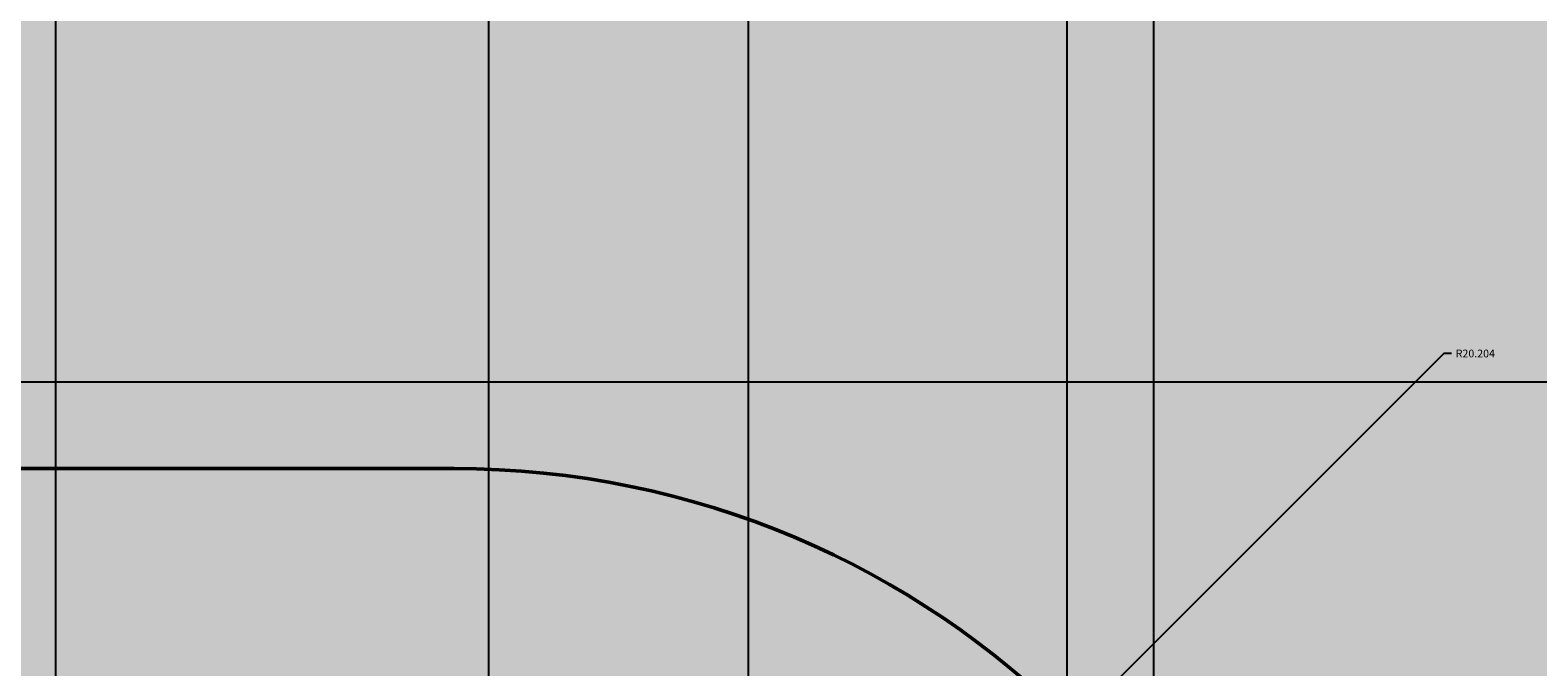
# Model space of a CAD drawing. Units: inches. Extents: x -12 to 334, y -10 to 186.
# Tile 56 of 77: x 222 to 257, y 96 to 111. Entities that reach past the tile are written whole.
import ezdxf

# ---------------------------------------------------------------- set-up
doc = ezdxf.new("R2010")
doc.units = ezdxf.units.IN
doc.header["$MEASUREMENT"] = 0
for name, color, linetype, lineweight in [('M-DIMS', 2, 'Continuous', 18), ('M-EQPM', 7, 'Continuous', 50), ('M-EQPM-PATT', 8, 'Continuous', 18)]:
    doc.layers.add(name, color=color, linetype=linetype, lineweight=lineweight)
doc.styles.get("Standard").update_dxf_attribs({"font": 'arial.ttf'})
doc.dimstyles.get("Standard").update_dxf_attribs({"dimtxt": 0.18, "dimasz": 0.18, "dimexe": 0.18, "dimexo": 0.0625, "dimgap": 0.09, "dimtad": 0, "dimtih": 1, "dimtoh": 1, "dimdec": 4, "dimzin": 0, "dimdsep": 46, "dimtxsty": 'Standard', "dimcen": 0.09, "dimadec": 0, "dimazin": 0, "dimtfac": 1, "dimtdec": 4, "dimtofl": 0, "dimtmove": 0, "dimatfit": 3, "dimfxl": 1, "dimtolj": 1, "dimtzin": 0, "dimarcsym": 0})

# ---------------------------------------------------------------- blocks, each defined once
blk = doc.blocks.new('*D17')
at = {"layer": 'Defpoints', "color": 0, "transparency": 16777216}
for p in [(106.177, 102.896), (105.892, 56.321), (295.976, 56.321)]:
    blk.add_point(p, dxfattribs=at)
at = {"layer": 'M-DIMS', "color": 0, "lineweight": -2, "transparency": 16777216}
for p, q in [((106.24, 102.896), (296.156, 102.896)), ((295.976, 102.716), (295.976, 79.79)), ((295.976, 56.501), (295.976, 79.426)), ((105.954, 56.321), (296.156, 56.321))]:
    blk.add_line(p, q, dxfattribs=at)
at = {"layer": 'M-DIMS', "color": 0, "transparency": 16777216}
for points in [[(295.946, 102.716), (296.006, 102.716), (295.976, 102.896)], [(295.946, 56.501), (296.006, 56.501), (295.976, 56.321)]]:
    blk.add_solid(points, dxfattribs=at)
at = {"layer": 'M-DIMS', "color": 0, "transparency": 16777216, "insert": (295.976, 79.608), "char_height": 0.18, "attachment_point": 5}
blk.add_mtext('\\A1;46.575', dxfattribs=at)
blk = doc.blocks.new('*D27')
at = {"layer": 'Defpoints', "color": 0, "transparency": 16777216}
for p in [(238.576, 169.385), (216.576, 32.854), (238.576, 32.854)]:
    blk.add_point(p, dxfattribs=at)
at = {"layer": 'M-DIMS', "color": 0, "lineweight": -2, "transparency": 16777216}
for p, q in [((216.576, 32.917), (216.576, 169.565)), ((238.576, 32.917), (238.576, 169.565)), ((216.756, 169.385), (227.357, 169.385)), ((238.396, 169.385), (227.796, 169.385))]:
    blk.add_line(p, q, dxfattribs=at)
at = {"layer": 'M-DIMS', "color": 0, "transparency": 16777216}
for points in [[(216.756, 169.415), (216.756, 169.355), (216.576, 169.385)], [(238.396, 169.415), (238.396, 169.355), (238.576, 169.385)]]:
    blk.add_solid(points, dxfattribs=at)
at = {"layer": 'M-DIMS', "color": 0, "transparency": 16777216, "insert": (227.576, 169.385), "char_height": 0.18, "attachment_point": 5}
blk.add_mtext('\\A1;22', dxfattribs=at)
blk = doc.blocks.new('*D28')
at = {"layer": 'Defpoints', "color": 0, "transparency": 16777216}
for p in [(232.576, 169.385), (222.576, 30.854), (232.576, 30.854)]:
    blk.add_point(p, dxfattribs=at)
at = {"layer": 'M-DIMS', "color": 0, "lineweight": -2, "transparency": 16777216}
for p, q in [((222.576, 30.917), (222.576, 169.565)), ((232.576, 30.917), (232.576, 169.565)), ((222.756, 169.385), (227.366, 169.385)), ((232.396, 169.385), (227.786, 169.385))]:
    blk.add_line(p, q, dxfattribs=at)
at = {"layer": 'M-DIMS', "color": 0, "transparency": 16777216}
for points in [[(222.756, 169.415), (222.756, 169.355), (222.576, 169.385)], [(232.396, 169.415), (232.396, 169.355), (232.576, 169.385)]]:
    blk.add_solid(points, dxfattribs=at)
at = {"layer": 'M-DIMS', "color": 0, "transparency": 16777216, "insert": (227.576, 169.385), "char_height": 0.18, "attachment_point": 5}
blk.add_mtext('\\A1;10', dxfattribs=at)
blk = doc.blocks.new('*D36')
at = {"layer": 'Defpoints', "color": 0, "transparency": 16777216}
for p in [(247.935, 169.385), (245.935, 82.697), (247.935, 82.697)]:
    blk.add_point(p, dxfattribs=at)
at = {"layer": 'M-DIMS', "color": 0, "lineweight": -2, "transparency": 16777216}
for p, q in [((245.935, 82.759), (245.935, 169.565)), ((247.935, 82.759), (247.935, 169.565)), ((246.115, 169.385), (246.786, 169.385)), ((247.755, 169.385), (247.085, 169.385))]:
    blk.add_line(p, q, dxfattribs=at)
at = {"layer": 'M-DIMS', "color": 0, "transparency": 16777216}
for points in [[(246.115, 169.415), (246.115, 169.355), (245.935, 169.385)], [(247.755, 169.415), (247.755, 169.355), (247.935, 169.385)]]:
    blk.add_solid(points, dxfattribs=at)
at = {"layer": 'M-DIMS', "color": 0, "transparency": 16777216, "insert": (246.935, 169.385), "char_height": 0.18, "attachment_point": 5}
blk.add_mtext('\\A1;2', dxfattribs=at)
blk = doc.blocks.new('*D37')
at = {"layer": 'Defpoints', "color": 0, "transparency": 16777216}
for p in [(245.935, 169.385), (232.576, 46.854), (245.935, 46.854)]:
    blk.add_point(p, dxfattribs=at)
at = {"layer": 'M-DIMS', "color": 0, "lineweight": -2, "transparency": 16777216}
for p, q in [((232.576, 46.917), (232.576, 169.565)), ((245.935, 46.917), (245.935, 169.565)), ((232.756, 169.385), (238.871, 169.385)), ((245.755, 169.385), (239.641, 169.385))]:
    blk.add_line(p, q, dxfattribs=at)
at = {"layer": 'M-DIMS', "color": 0, "transparency": 16777216}
for points in [[(232.756, 169.415), (232.756, 169.355), (232.576, 169.385)], [(245.755, 169.415), (245.755, 169.355), (245.935, 169.385)]]:
    blk.add_solid(points, dxfattribs=at)
at = {"layer": 'M-DIMS', "color": 0, "transparency": 16777216, "insert": (239.256, 169.385), "char_height": 0.18, "attachment_point": 5}
blk.add_mtext('\\A1;13.36', dxfattribs=at)
blk = doc.blocks.new('*D40')
at = {"layer": 'Defpoints', "color": 0, "transparency": 16777216}
for p in [(278.229, 116.208), (187.394, 91.899)]:
    blk.add_point(p, dxfattribs=at)
at = {"layer": 'M-DIMS', "color": 0, "lineweight": -2, "transparency": 16777216}
for p, q in [((332.73, 130.793), (278.403, 116.254)), ((187.394, 91.809), (187.394, 91.989)), ((187.304, 91.899), (187.484, 91.899))]:
    blk.add_line(p, q, dxfattribs=at)
at = {"layer": 'M-DIMS', "color": 0, "transparency": 16777216}
blk.add_solid([(278.395, 116.283), (278.411, 116.225), (278.229, 116.208)], dxfattribs=at)
at = {"layer": 'M-DIMS', "color": 0, "transparency": 16777216, "insert": (333.21, 130.793), "char_height": 0.18, "attachment_point": 5}
blk.add_mtext('\\A1;R94.03', dxfattribs=at)
blk = doc.blocks.new('*D43')
at = {"layer": 'Defpoints', "color": 0, "transparency": 16777216}
for p in [(246.06, 94.98), (231.776, 80.692)]:
    blk.add_point(p, dxfattribs=at)
at = {"layer": 'M-DIMS', "color": 0, "lineweight": -2, "transparency": 16777216}
for p, q in [((254.631, 103.553), (246.187, 95.108)), ((254.811, 103.553), (254.631, 103.553)), ((231.776, 80.602), (231.776, 80.782)), ((231.686, 80.692), (231.866, 80.692))]:
    blk.add_line(p, q, dxfattribs=at)
at = {"layer": 'M-DIMS', "color": 0, "transparency": 16777216}
blk.add_solid([(246.166, 95.129), (246.209, 95.086), (246.06, 94.98)], dxfattribs=at)
at = {"layer": 'M-DIMS', "color": 0, "transparency": 16777216, "insert": (255.36, 103.553), "char_height": 0.18, "attachment_point": 5}
blk.add_mtext('\\A1;R20.204', dxfattribs=at)

msp = doc.modelspace()

# ---------------------------------------------------------------- hatches: boundary and pattern name
at = {"layer": 'M-EQPM-PATT', "transparency": 33554556}
h = msp.add_hatch(color=256, dxfattribs=at)
h.set_gradient(color1=(248, 206, 179), color2=(248, 206, 179), tint=1)
h.paths.add_polyline_path([(179.7818, 136.8871), (126.9567, 136.8871), (106.1771, 100.8958), (171.5458, 100.8958)])
h.paths.add_polyline_path([(268.3808, 136.9435), (214.0166, 136.9435), (214.0166, 154.8345), (196.3421, 154.8345), (196.3421, 136.8871), (179.7818, 136.8871), (171.5458, 100.8958), (231.7758, 100.8958, -0.4142136), (251.9801, 80.6915), (279.7263, 80.6915, 0.1631825)])
at = {"layer": 'M-EQPM-PATT'}
h = msp.add_hatch(color=256, dxfattribs=at)
h.set_gradient(color1=(94, 103, 175), color2=(94, 103, 175), tint=1)
h.paths.add_polyline_path([(129.093, 89.8963), (86.8879, 89.8963), (86.8879, 69.6117), (129.093, 69.6117)], flags=17)
h.paths.add_polyline_path([(170.9079, 89.8963), (130.8573, 89.8963), (130.8573, 69.6117), (170.9079, 69.6117)], flags=17)
h.paths.add_polyline_path([(216.4278, 89.8963), (172.6722, 89.8963), (172.6722, 69.6117), (216.4278, 69.6117)], flags=17)
h.paths.add_polyline_path([(245.9354, 82.6969), (247.9354, 82.6969), (247.9354, 46.8541), (268.3808, 46.8541, 0.0998398), (279.7263, 80.6915), (251.9801, 80.6915, 0.4142136), (231.7758, 100.8958), (84.7229, 100.8958), (84.7229, 109.0583), (83.7229, 109.0583), (83.7229, 95.8963), (129.093, 95.8963), (129.093, 98.1081), (130.8573, 98.1081), (130.8573, 95.8963), (170.9079, 95.8963), (170.9079, 98.1081), (172.6722, 98.1081), (172.6722, 95.8963), (216.4278, 95.8963), (216.4278, 98.1081), (218.1922, 98.1081), (218.1922, 95.8963), (226.6083, 95.8963, -1), (226.6083, 63.6117), (218.1922, 63.6117), (218.1922, 61.1045), (216.4278, 61.1045), (216.4278, 63.6117), (172.6722, 63.6117), (172.6722, 61.1045), (170.9079, 61.1045), (170.9079, 63.6117), (130.8573, 63.6117), (130.8573, 61.1045), (129.093, 61.1045), (129.093, 63.6117), (87.8879, 63.6117), (87.8879, 56.3205), (105.8919, 56.3205), (105.8919, 28.8541), (115.8919, 28.8541), (115.8919, 46.8541), (222.5761, 46.8541), (222.5761, 30.8541), (232.5761, 30.8541), (232.5761, 46.8541), (245.9354, 46.8541)])
h.paths.add_polyline_path([(86.8879, 89.8963), (75.9244, 89.8963), (75.9244, 69.6117), (86.8879, 69.6117)])
h.paths.add_polyline_path([(83.7229, 109.0583), (75.9244, 109.0583), (75.9244, 95.8963), (83.7229, 95.8963)])
h.paths.add_polyline_path([(226.6083, 89.8963), (218.1922, 89.8963), (218.1922, 69.6117), (226.6083, 69.6117, 1)], flags=17)
h = msp.add_hatch(color=256, dxfattribs=at)
h.set_gradient(color1=(0, 0, 255), color2=(0, 0, 255), tint=1)
h.paths.add_polyline_path([(84.7229, 100.8958), (84.7229, 109.0583), (83.7229, 109.0583), (83.7229, 95.8963), (129.093, 95.8963), (129.093, 98.1081), (130.8573, 98.1081), (130.8573, 95.8963), (170.9079, 95.8963), (170.9079, 98.1081), (172.6722, 98.1081), (172.6722, 95.8963), (216.4278, 95.8963), (216.4278, 98.1081), (218.1922, 98.1081), (218.1922, 95.8963), (226.6083, 95.8963, -1), (226.6083, 63.6117), (218.1922, 63.6117), (218.1922, 61.1045), (216.4278, 61.1045), (216.4278, 63.6117), (172.6722, 63.6117), (172.6722, 61.1045), (170.9079, 61.1045), (170.9079, 63.6117), (130.8573, 63.6117), (130.8573, 61.1045), (129.093, 61.1045), (129.093, 63.6117), (87.8879, 63.6117), (87.8879, 56.3205), (105.8919, 56.3205), (105.8919, 28.8541), (115.8919, 28.8541), (115.8919, 46.8541), (222.5761, 46.8541), (222.5761, 30.8541), (232.5761, 30.8541), (232.5761, 46.8541), (245.9354, 46.8541), (245.9354, 82.6969), (247.9354, 82.6969), (247.9354, 46.8541), (268.3808, 46.8541, 0.0998398), (279.7263, 80.6915), (251.9801, 80.6915, 0.4142136), (231.7758, 100.8958)])

# ---------------------------------------------------------------- linework, layer by layer
at = {"layer": 'M-EQPM'}
msp.add_lwpolyline([(84.7229, 100.8958), (231.7758, 100.8958)], dxfattribs=at)
msp.add_arc((231.7758, 80.6915), 20.2043, 0, 90, dxfattribs=at)

# ---------------------------------------------------------------- dimensions: what is measured, and where the dimension line sits
at = {"layer": 'M-DIMS'}
for base, p1, p2, override, picture, middle in [((238.5761, 169.3845), (216.5761, 32.8541), (238.5761, 32.8541), {"dimdec": 0, "dimlfac": 1, "dimrnd": 0, "dimzin": 0, "dimdsep": 46, "dimlunit": 2}, '*D27', (227.5761, 169.3845)), ((232.5761, 169.3845), (222.5761, 30.8541), (232.5761, 30.8541), {"dimdec": 0, "dimlfac": 1, "dimrnd": 0, "dimzin": 0, "dimdsep": 46, "dimlunit": 2}, '*D28', (227.5761, 169.3845)), ((245.9354, 169.3845), (232.5761, 46.8541), (245.9354, 46.8541), {"dimdec": 2, "dimlfac": 1, "dimrnd": 0, "dimzin": 0, "dimdsep": 46, "dimlunit": 2}, '*D37', (239.2558, 169.3845)), ((247.9354, 169.3845), (245.9354, 82.6969), (247.9354, 82.6969), {"dimdec": 0, "dimlfac": 1, "dimrnd": 0, "dimzin": 0, "dimdsep": 46, "dimlunit": 2}, '*D36', (246.9354, 169.3845))]:
    dim = msp.add_linear_dim(base=base, p1=p1, p2=p2, dimstyle='Standard', override=override, dxfattribs=at)
    dim.commit()
    dim.dimension.update_dxf_attribs({"geometry": picture, "text_midpoint": middle})
for center, mpoint, override, picture, middle in [((187.3936, 91.8988), (278.2291, 116.2078), {"dimdec": 2, "dimlfac": 1, "dimrnd": 0, "dimzin": 0, "dimdsep": 46, "dimlunit": 2}, '*D40', (332.7304, 130.7932)), ((231.7758, 80.6915), (246.0602, 94.9802), {"dimdec": 3, "dimlfac": 1, "dimrnd": 0, "dimzin": 0, "dimdsep": 46, "dimlunit": 2}, '*D43', (255.3603, 103.5535))]:
    dim = msp.add_radius_dim(center=center, mpoint=mpoint, dimstyle='Standard', override=override, dxfattribs=at)
    dim.commit()
    dim.dimension.update_dxf_attribs({"geometry": picture, "text_midpoint": middle, "dimtype": 164})
dim = msp.add_linear_dim(base=(295.9756, 56.3205), p1=(106.1771, 102.8958), p2=(105.8919, 56.3205), angle=90, dimstyle='Standard', override={"dimdec": 3, "dimlfac": 1, "dimrnd": 0, "dimzin": 0, "dimdsep": 46, "dimlunit": 2}, dxfattribs=at)
dim.commit()
dim.dimension.update_dxf_attribs({"geometry": '*D17', "text_midpoint": (295.9756, 79.6082)})

doc.saveas('drawing.dxf')
